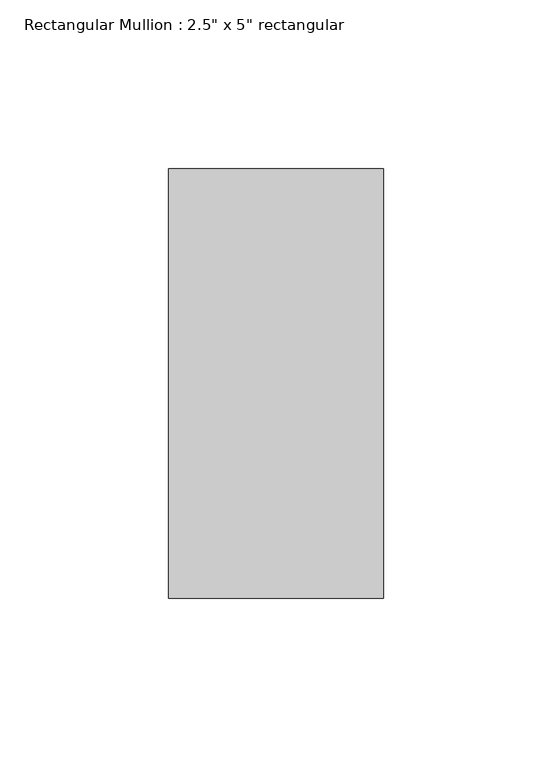
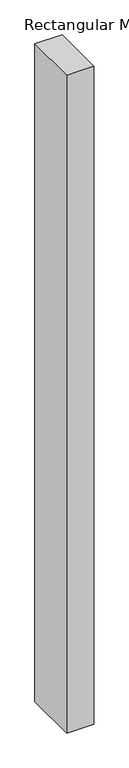
"""IFC4 building model written with IfcOpenShell, lengths in millimetres: member geometry."""

from ifc_helpers import new_model, si_unit, frame, origin, place, context, project, spatial, polyline, outline, extrude, source, transform, mapped, element, save


def member_2dc5f12d(model_context):
    return source(origin(), model_context, "Body", "SweptSolid", [
        extrude(outline(polyline([(0.0, 63.5), (0.0, -63.5), (-63.5, -63.5), (-63.5, 63.5), (0.0, 63.5)])), frame((0.0, 0.0, -1611.1494203), z_axis=(0.0, 0.0, 1.0), x_axis=(1.0, 0.0, 0.0)), (0.0, 0.0, 1.0), 1611.1494203),
    ])


if __name__ == "__main__":
    model = new_model("IFC4")
    model_context = context("Model", 3, world=origin())
    ifc_project = project(units=[si_unit("LENGTHUNIT", "METRE", prefix="MILLI")], contexts=[model_context])
    site = spatial("IfcSite", under=ifc_project)
    building = spatial("IfcBuilding", under=site)
    placement = place(None, origin())
    member_shape = member_2dc5f12d(model_context)
    element("IfcMember", 1, ObjectType="Rectangular Mullion : 2.5\" x 5\" rectangular", at=placement, inside=building, context=model_context, shape_type="MappedRepresentation", body=[
        mapped(member_shape, transform((0.0, 0.0, 0.0), x_axis=(1.0, 0.0, 0.0), y_axis=(0.0, 1.0, 0.0), z_axis=(0.0, 0.0, 1.0))),
    ])
    save(model, "model.ifc")

# Revit data of these elements
# Type "Rectangular Mullion : 2.5\" x 5\" rectangular"
#   built-in parameter 1007304 = 0.416667 (stored number, unit not read)
#   built-in parameter 1007301 = 0.104167 (stored number, unit not read)
#   built-in parameter 1007300 = 0.104167 (stored number, unit not read)
# Element 1 (IfcMember, "Rectangular Mullion : 2.5\" x 5\" rectangular")
#   Materials on its faces: "Aluminum"
# Materials
#   "Aluminum": class "Metal", colour RGB 247 247 247, transparency 0, Description = "Aluminum 6061", Cost = 0
